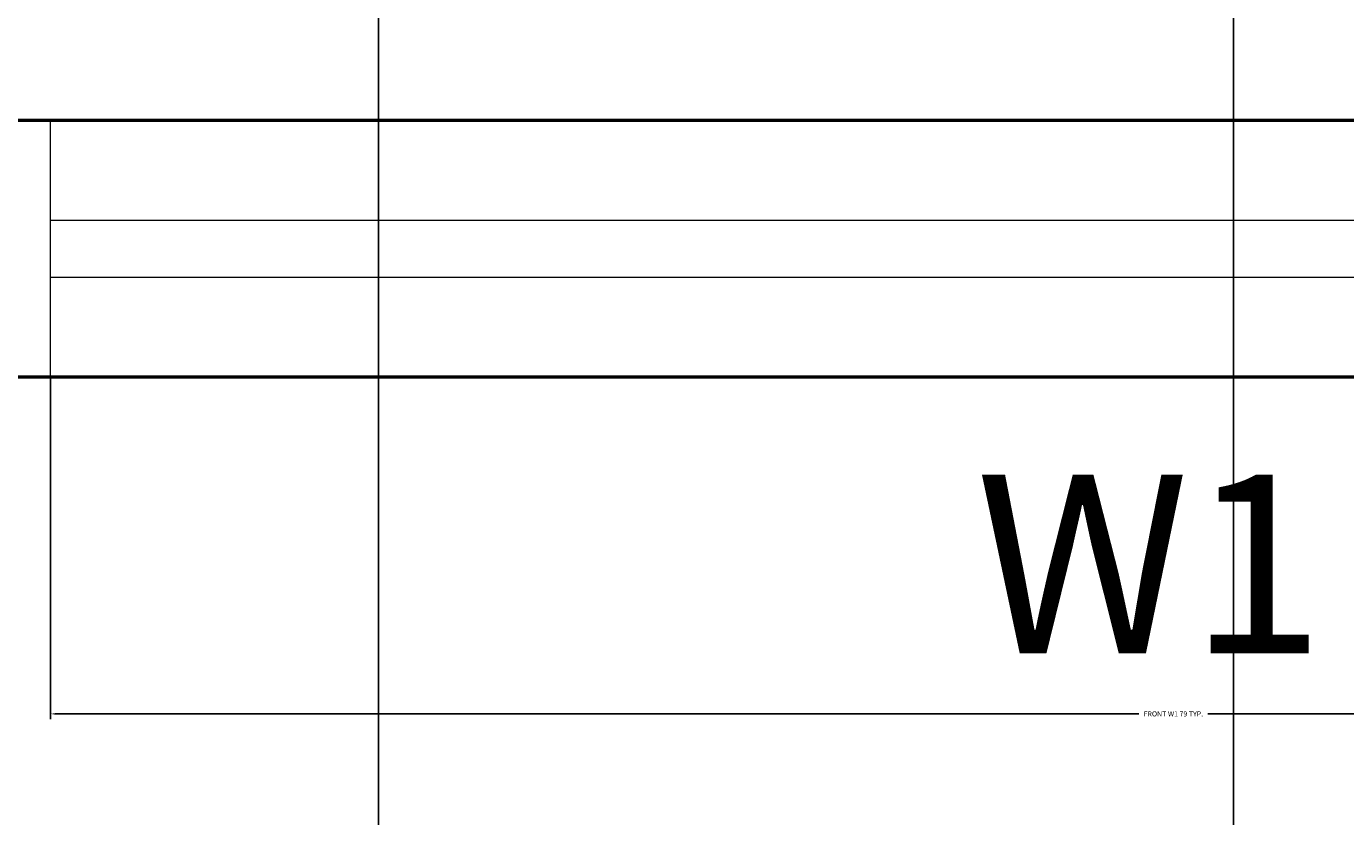
# Model space of a CAD drawing. Units: inches. Extents: x 7359 to 7979, y 33027 to 34263.
# Tile 23 of 32: x 7550 to 7597, y 33749 to 33777. Entities that reach past the tile are written whole.
import ezdxf

# ---------------------------------------------------------------- set-up
doc = ezdxf.new("R2010")
doc.units = ezdxf.units.IN
for name, color, linetype, lineweight in [('A-ANNO-DIMS', 2, 'Continuous', 18), ('A-ANNO-TEXT', 3, 'Continuous', 18), ('A-GLAZ', 4, 'Continuous', 18), ('A-WALL', 7, 'Continuous', 50)]:
    doc.layers.add(name, color=color, linetype=linetype, lineweight=lineweight)
doc.styles.get("Standard").update_dxf_attribs({"font": 'arial.ttf'})
doc.dimstyles.get("Standard").update_dxf_attribs({"dimtxt": 0.18, "dimasz": 0.18, "dimexe": 0.18, "dimexo": 0.0625, "dimgap": 0.09, "dimtad": 0, "dimtih": 1, "dimtoh": 1, "dimdec": 4, "dimzin": 0, "dimdsep": 46, "dimtxsty": 'Standard', "dimcen": 0.09, "dimadec": 0, "dimazin": 0, "dimtfac": 1, "dimtdec": 4, "dimtofl": 0, "dimtmove": 0, "dimatfit": 3, "dimfxl": 1, "dimtolj": 1, "dimtzin": 0, "dimarcsym": 0})

# ---------------------------------------------------------------- blocks, each defined once
blk = doc.blocks.new('WINDOW-W1-DRAWING-FRONT')
for p, q in [((0, 0), (0, 9)), ((0, 5.5), (78.794, 5.5)), ((0, 3.5), (78.794, 3.5))]:
    blk.add_line(p, q)
blk = doc.blocks.new('*D62')
at = {"layer": 'A-ANNO-DIMS', "color": 0, "lineweight": -2, "transparency": 16777216}
for p, q in [((7551.084, 33764.771), (7551.084, 33752.835)), ((7629.878, 33764.771), (7629.878, 33752.835)), ((7551.264, 33753.015), (7589.266, 33753.015)), ((7629.698, 33753.015), (7591.695, 33753.015))]:
    blk.add_line(p, q, dxfattribs=at)
at = {"layer": 'A-ANNO-DIMS', "color": 0, "transparency": 16777216}
for points in [[(7551.264, 33753.045), (7551.264, 33752.985), (7551.084, 33753.015)], [(7629.698, 33753.045), (7629.698, 33752.985), (7629.878, 33753.015)]]:
    blk.add_solid(points, dxfattribs=at)
at = {"layer": 'Defpoints', "color": 0, "transparency": 16777216}
for p in [(7551.084, 33764.834), (7629.878, 33764.834), (7629.878, 33753.015)]:
    blk.add_point(p, dxfattribs=at)
at = {"layer": 'A-ANNO-DIMS', "color": 0, "transparency": 16777216, "insert": (7590.481, 33753.015), "char_height": 0.18, "attachment_point": 5}
blk.add_mtext('\\A1;FRONT W1 79 TYP.', dxfattribs=at)
blk = doc.blocks.new('*D68')
at = {"layer": 'A-ANNO-DIMS', "color": 0, "lineweight": -2, "transparency": 16777216}
for p, q in [((7562.591, 34181.771), (7562.591, 33632.309)), ((7592.591, 34181.771), (7592.591, 33632.309)), ((7562.771, 33632.489), (7577.373, 33632.489)), ((7592.411, 33632.489), (7577.81, 33632.489))]:
    blk.add_line(p, q, dxfattribs=at)
at = {"layer": 'A-ANNO-DIMS', "color": 0, "transparency": 16777216}
for points in [[(7562.771, 33632.519), (7562.771, 33632.459), (7562.591, 33632.489)], [(7592.411, 33632.519), (7592.411, 33632.459), (7592.591, 33632.489)]]:
    blk.add_solid(points, dxfattribs=at)
at = {"layer": 'Defpoints', "color": 0, "transparency": 16777216}
for p in [(7562.591, 34181.834), (7592.591, 34181.834), (7592.591, 33632.489)]:
    blk.add_point(p, dxfattribs=at)
at = {"layer": 'A-ANNO-DIMS', "color": 0, "transparency": 16777216, "insert": (7577.591, 33632.489), "char_height": 0.18, "attachment_point": 5}
blk.add_mtext('\\A1;30', dxfattribs=at)
blk = doc.blocks.new('*D83')
at = {"layer": 'A-ANNO-DIMS', "color": 0, "lineweight": -2, "transparency": 16777216}
for p, q in [((7592.591484, 34081.771428), (7592.591484, 33632.309146)), ((7598.591484, 34081.771428), (7598.591484, 33632.309146)), ((7592.771484, 33632.489146), (7595.442057, 33632.489146)), ((7598.411484, 33632.489146), (7595.740911, 33632.489146))]:
    blk.add_line(p, q, dxfattribs=at)
at = {"layer": 'A-ANNO-DIMS', "color": 0, "transparency": 16777216}
for points in [[(7592.771484, 33632.519146), (7592.771484, 33632.459146), (7592.591484, 33632.489146)], [(7598.411484, 33632.519146), (7598.411484, 33632.459146), (7598.591484, 33632.489146)]]:
    blk.add_solid(points, dxfattribs=at)
at = {"layer": 'Defpoints', "color": 0, "transparency": 16777216}
for p in [(7592.591484, 34081.833928), (7598.591484, 34081.833928), (7598.591484, 33632.489146)]:
    blk.add_point(p, dxfattribs=at)
at = {"layer": 'A-ANNO-DIMS', "color": 0, "transparency": 16777216, "insert": (7595.591484, 33632.489146), "char_height": 0.18, "attachment_point": 5}
blk.add_mtext('\\A1;6', dxfattribs=at)

msp = doc.modelspace()

# ---------------------------------------------------------------- linework, layer by layer
at = {"layer": 'A-WALL'}
for p, q in [((7467.5915, 33773.8339), (7689.4915, 33773.8339)), ((7458.5915, 33764.8339), (7883.9915, 33764.8339))]:
    msp.add_line(p, q, dxfattribs=at)

# ---------------------------------------------------------------- block references
at = {"layer": 'A-GLAZ'}
msp.add_blockref('WINDOW-W1-DRAWING-FRONT', (7551.084, 33764.834), dxfattribs=at)

# ---------------------------------------------------------------- texts
at = {"layer": 'A-ANNO-TEXT'}
msp.add_text('W1', height=6.25941, dxfattribs=at).set_placement((7583.5421, 33755.1433))

# ---------------------------------------------------------------- dimensions: what is measured, and where the dimension line sits
at = {"layer": 'A-ANNO-DIMS'}
for base, p1, p2, picture, middle in [((7592.5915, 33632.4891), (7562.5915, 34181.8339), (7592.5915, 34181.8339), '*D68', (7577.5915, 33632.4891)), ((7598.5915, 33632.4891), (7592.5915, 34081.8339), (7598.5915, 34081.8339), '*D83', (7595.5915, 33632.4891))]:
    dim = msp.add_linear_dim(base=base, p1=p1, p2=p2, dimstyle='Standard', override={"dimdec": 0, "dimlfac": 1, "dimrnd": 0, "dimzin": 0, "dimdsep": 46, "dimlunit": 2}, dxfattribs=at)
    dim.commit()
    dim.dimension.update_dxf_attribs({"geometry": picture, "text_midpoint": middle})
dim = msp.add_linear_dim(base=(7629.8778, 33753.0149), p1=(7551.0841, 33764.8339), p2=(7629.8778, 33764.8339), text='FRONT W1 <> TYP.', dimstyle='Standard', override={"dimdec": 0, "dimlfac": 1, "dimrnd": 0, "dimzin": 0, "dimdsep": 46, "dimlunit": 2}, dxfattribs=at)
dim.commit()
dim.dimension.update_dxf_attribs({"geometry": '*D62', "text_midpoint": (7590.4809, 33753.0149)})

doc.saveas('drawing.dxf')
